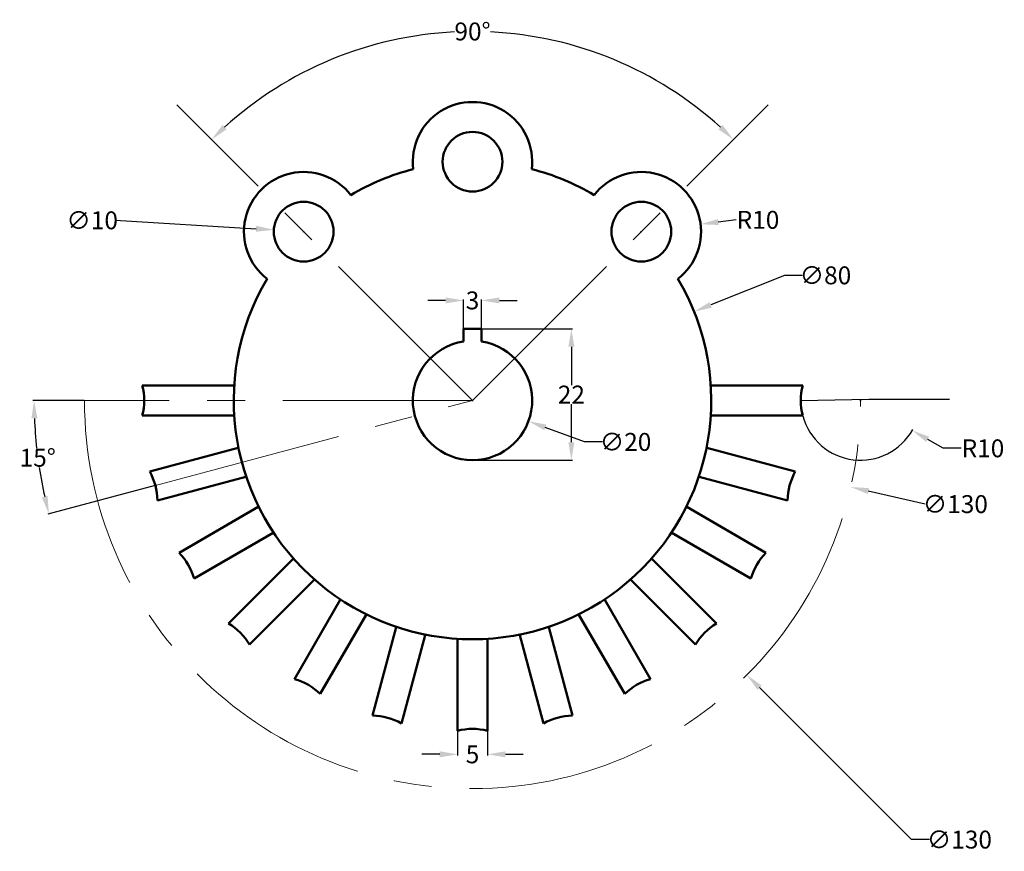
# Model space of a CAD drawing. Units: millimetres. Extents: x 201 to 366, y 129 to 269.
import ezdxf

# ---------------------------------------------------------------- set-up
doc = ezdxf.new("R2010")
doc.units = ezdxf.units.MM
doc.header["$MEASUREMENT"] = 0
doc.linetypes.add('CENTER', pattern=[50.8, 31.75, -6.35, 6.35, -6.35])
for name, color, linetype, lineweight in [('M-CNTR', 1, 'CENTER', 18), ('M-DIMS', 2, 'Continuous', 25), ('M-OUTL', 7, 'Continuous', 50)]:
    doc.layers.add(name, color=color, linetype=linetype, lineweight=lineweight)
doc.styles.get("Standard").update_dxf_attribs({"font": 'arial.ttf'})
doc.dimstyles.get("Standard").update_dxf_attribs({"dimtxt": 3, "dimasz": 3, "dimexe": 0.18, "dimexo": 0.0625, "dimgap": 0.09, "dimtad": 0, "dimtih": 1, "dimtoh": 1, "dimdec": 3, "dimdsep": 46, "dimtxsty": 'Standard', "dimcen": 0.09, "dimadec": 0, "dimazin": 0, "dimtfac": 1, "dimtdec": 3, "dimtofl": 0, "dimtmove": 0, "dimatfit": 3, "dimfxl": 1, "dimtolj": 1, "dimtzin": 0, "dimarcsym": 0})

# ---------------------------------------------------------------- blocks, each defined once
blk = doc.blocks.new('*D1')
at = {"layer": 'Defpoints', "color": 0, "transparency": 16777216}
for p in [(211.72, 204.93), (276.72, 204.93), (276.72, 204.93), (203.54, 198.53), (223.59, 190.7)]:
    blk.add_point(p, dxfattribs=at)
at = {"layer": 'M-DIMS', "color": 0, "lineweight": -2, "transparency": 16777216}
for p, q in [((211.65, 204.93), (203.08, 204.93)), ((223.53, 190.68), (205.59, 185.87))]:
    blk.add_line(p, q, dxfattribs=at)
for start, end in [(182.34, 186.226), (188.7777, 192.66)]:
    blk.add_arc((276.72, 204.93), 73.46, start, end, dxfattribs=at)
at = {"layer": 'M-DIMS', "color": 0, "transparency": 16777216}
for points in [[(202.82, 201.92), (203.82, 201.95), (203.26, 204.93)], [(205.53, 188.95), (204.56, 188.71), (205.76, 185.92)]]:
    blk.add_solid(points, dxfattribs=at)
at = {"layer": 'M-DIMS', "color": 0, "transparency": 16777216, "insert": (203.88, 195.35), "char_height": 3, "attachment_point": 5}
blk.add_mtext('\\A1;15°', dxfattribs=at)
blk = doc.blocks.new('*D2')
at = {"layer": 'Defpoints', "color": 0, "transparency": 16777216}
for p in [(213.35, 219.43), (340.08, 190.44)]:
    blk.add_point(p, dxfattribs=at)
at = {"layer": 'M-DIMS', "color": 0, "lineweight": -2, "transparency": 16777216}
for p, q in [((276.63, 204.93), (276.81, 204.93)), ((276.72, 204.84), (276.72, 205.02)), ((352.57, 187.58), (343, 189.77))]:
    blk.add_line(p, q, dxfattribs=at)
at = {"layer": 'M-DIMS', "color": 0, "transparency": 16777216}
blk.add_solid([(343.12, 190.26), (342.89, 189.28), (340.08, 190.44)], dxfattribs=at)
at = {"layer": 'M-DIMS', "color": 0, "transparency": 16777216, "insert": (357.61, 187.58), "char_height": 3, "attachment_point": 5}
blk.add_mtext('\\A1;∅130', dxfattribs=at)
blk = doc.blocks.new('*D3')
at = {"layer": 'Defpoints', "color": 0, "transparency": 16777216}
for p in [(341.72, 204.93), (350.38, 199.93)]:
    blk.add_point(p, dxfattribs=at)
at = {"layer": 'M-DIMS', "color": 0, "lineweight": -2, "transparency": 16777216}
for p, q in [((341.63, 204.93), (341.81, 204.93)), ((341.72, 204.84), (341.72, 205.02)), ((355.57, 196.93), (352.98, 198.43)), ((358.57, 196.93), (355.57, 196.93))]:
    blk.add_line(p, q, dxfattribs=at)
blk.add_arc((341.72, 204.93), 10, 194.8356, 331.0313, dxfattribs=at)
at = {"layer": 'M-DIMS', "color": 0, "transparency": 16777216}
blk.add_solid([(353.23, 198.87), (352.73, 198), (350.38, 199.93)], dxfattribs=at)
at = {"layer": 'M-DIMS', "color": 0, "transparency": 16777216, "insert": (362.24, 196.93), "char_height": 3, "attachment_point": 5}
blk.add_mtext('\\A1;R10', dxfattribs=at)
blk = doc.blocks.new('*D4')
at = {"layer": 'Defpoints', "color": 0, "transparency": 16777216}
for p in [(274.22, 149.62), (279.22, 149.62), (279.22, 145.67)]:
    blk.add_point(p, dxfattribs=at)
at = {"layer": 'M-DIMS', "color": 0, "lineweight": -2, "transparency": 16777216}
for p, q in [((274.22, 149.55), (274.22, 145.49)), ((279.22, 149.55), (279.22, 145.49)), ((271.22, 145.67), (268.22, 145.67)), ((282.22, 145.67), (285.22, 145.67))]:
    blk.add_line(p, q, dxfattribs=at)
at = {"layer": 'M-DIMS', "color": 0, "transparency": 16777216}
for points in [[(271.22, 146.17), (271.22, 145.17), (274.22, 145.67)], [(282.22, 146.17), (282.22, 145.17), (279.22, 145.67)]]:
    blk.add_solid(points, dxfattribs=at)
at = {"layer": 'M-DIMS', "color": 0, "transparency": 16777216, "insert": (276.72, 145.67), "char_height": 3, "attachment_point": 5}
blk.add_mtext('\\A1;5', dxfattribs=at)
blk = doc.blocks.new('*D5')
at = {"layer": 'Defpoints', "color": 0, "transparency": 16777216}
for p in [(292.72, 264.65), (227.18, 254.47), (326.25, 254.47), (276.72, 204.93), (276.72, 204.93)]:
    blk.add_point(p, dxfattribs=at)
at = {"layer": 'M-DIMS', "color": 0, "lineweight": -2, "transparency": 16777216}
for start, end in [(92.812, 132.2192), (47.7808, 87.188)]:
    blk.add_arc((276.72, 204.93), 61.82, start, end, dxfattribs=at)
at = {"layer": 'M-DIMS', "color": 0, "transparency": 16777216}
for points in [[(235.52, 250.35), (234.83, 251.08), (233.01, 248.65)], [(318.6, 251.08), (317.91, 250.35), (320.43, 248.65)]]:
    blk.add_solid(points, dxfattribs=at)
at = {"layer": 'M-DIMS', "color": 0, "transparency": 16777216, "insert": (276.72, 266.75), "char_height": 3, "attachment_point": 5}
blk.add_mtext('\\A1;90°', dxfattribs=at)
blk = doc.blocks.new('*D6')
at = {"layer": 'Defpoints', "color": 0, "transparency": 16777216}
for p in [(313.84, 219.83), (239.59, 190.04)]:
    blk.add_point(p, dxfattribs=at)
at = {"layer": 'M-DIMS', "color": 0, "lineweight": -2, "transparency": 16777216}
for p, q in [((328.99, 225.9), (316.63, 220.94)), ((331.99, 225.9), (328.99, 225.9)), ((276.63, 204.93), (276.81, 204.93)), ((276.72, 204.84), (276.72, 205.02))]:
    blk.add_line(p, q, dxfattribs=at)
at = {"layer": 'M-DIMS', "color": 0, "transparency": 16777216}
blk.add_solid([(316.44, 221.41), (316.81, 220.48), (313.84, 219.83)], dxfattribs=at)
at = {"layer": 'M-DIMS', "color": 0, "transparency": 16777216, "insert": (335.85, 225.9), "char_height": 3, "attachment_point": 5}
blk.add_mtext('\\A1;∅80', dxfattribs=at)
blk = doc.blocks.new('*D7')
at = {"layer": 'Defpoints', "color": 0, "transparency": 16777216}
for p in [(314.92, 234.46), (305, 233.22)]:
    blk.add_point(p, dxfattribs=at)
at = {"layer": 'M-DIMS', "color": 0, "lineweight": -2, "transparency": 16777216}
for p, q in [((320.88, 235.2), (317.9, 234.83)), ((304.91, 233.22), (305.09, 233.22)), ((305, 233.13), (305, 233.31))]:
    blk.add_line(p, q, dxfattribs=at)
at = {"layer": 'M-DIMS', "color": 0, "transparency": 16777216}
blk.add_solid([(317.84, 235.32), (317.96, 234.33), (314.92, 234.46)], dxfattribs=at)
at = {"layer": 'M-DIMS', "color": 0, "transparency": 16777216, "insert": (324.55, 235.2), "char_height": 3, "attachment_point": 5}
blk.add_mtext('\\A1;R10', dxfattribs=at)
blk = doc.blocks.new('*D8')
at = {"layer": 'Defpoints', "color": 0, "transparency": 16777216}
for p in [(243.44, 233.52), (253.42, 232.92)]:
    blk.add_point(p, dxfattribs=at)
at = {"layer": 'M-DIMS', "color": 0, "lineweight": -2, "transparency": 16777216}
for p, q in [((216.87, 235.12), (240.45, 233.7)), ((248.34, 233.22), (248.52, 233.22)), ((248.43, 233.13), (248.43, 233.31))]:
    blk.add_line(p, q, dxfattribs=at)
at = {"layer": 'M-DIMS', "color": 0, "transparency": 16777216}
blk.add_solid([(240.48, 234.2), (240.42, 233.2), (243.44, 233.52)], dxfattribs=at)
at = {"layer": 'M-DIMS', "color": 0, "transparency": 16777216, "insert": (213, 235.12), "char_height": 3, "attachment_point": 5}
blk.add_mtext('\\A1;∅10', dxfattribs=at)
blk = doc.blocks.new('*D9')
at = {"layer": 'Defpoints', "color": 0, "transparency": 16777216}
for p in [(267.34, 208.4), (286.1, 201.47)]:
    blk.add_point(p, dxfattribs=at)
at = {"layer": 'M-DIMS', "color": 0, "lineweight": -2, "transparency": 16777216}
for p, q in [((276.63, 204.93), (276.81, 204.93)), ((276.72, 204.84), (276.72, 205.02)), ((295.49, 198), (288.91, 200.43)), ((298.49, 198), (295.49, 198))]:
    blk.add_line(p, q, dxfattribs=at)
at = {"layer": 'M-DIMS', "color": 0, "transparency": 16777216}
blk.add_solid([(289.09, 200.9), (288.74, 199.96), (286.1, 201.47)], dxfattribs=at)
at = {"layer": 'M-DIMS', "color": 0, "transparency": 16777216, "insert": (302.36, 198), "char_height": 3, "attachment_point": 5}
blk.add_mtext('\\A1;∅20', dxfattribs=at)
blk = doc.blocks.new('*D10')
at = {"layer": 'Defpoints', "color": 0, "transparency": 16777216}
for p in [(278.22, 221.7), (275.22, 216.93), (278.22, 216.93)]:
    blk.add_point(p, dxfattribs=at)
at = {"layer": 'M-DIMS', "color": 0, "lineweight": -2, "transparency": 16777216}
for p, q in [((272.22, 221.7), (269.22, 221.7)), ((275.22, 217), (275.22, 221.88)), ((278.22, 217), (278.22, 221.88)), ((281.22, 221.7), (284.22, 221.7))]:
    blk.add_line(p, q, dxfattribs=at)
at = {"layer": 'M-DIMS', "color": 0, "transparency": 16777216}
for points in [[(272.22, 222.2), (272.22, 221.2), (275.22, 221.7)], [(281.22, 222.2), (281.22, 221.2), (278.22, 221.7)]]:
    blk.add_solid(points, dxfattribs=at)
at = {"layer": 'M-DIMS', "color": 0, "transparency": 16777216, "insert": (276.72, 221.7), "char_height": 3, "attachment_point": 5}
blk.add_mtext('\\A1;3', dxfattribs=at)
blk = doc.blocks.new('*D11')
at = {"layer": 'Defpoints', "color": 0, "transparency": 16777216}
for p in [(276.71, 216.93), (276.72, 194.93), (293.28, 194.93)]:
    blk.add_point(p, dxfattribs=at)
at = {"layer": 'M-DIMS', "color": 0, "lineweight": -2, "transparency": 16777216}
for p, q in [((276.77, 216.93), (293.46, 216.93)), ((293.28, 213.93), (293.28, 207.53)), ((293.28, 197.93), (293.28, 204.34)), ((276.79, 194.93), (293.46, 194.93))]:
    blk.add_line(p, q, dxfattribs=at)
at = {"layer": 'M-DIMS', "color": 0, "transparency": 16777216}
for points in [[(292.78, 213.93), (293.78, 213.93), (293.28, 216.93)], [(292.78, 197.93), (293.78, 197.93), (293.28, 194.93)]]:
    blk.add_solid(points, dxfattribs=at)
at = {"layer": 'M-DIMS', "color": 0, "transparency": 16777216, "insert": (293.28, 205.93), "char_height": 3, "attachment_point": 5}
blk.add_mtext('\\A1;22', dxfattribs=at)
blk = doc.blocks.new('*D12')
at = {"layer": 'Defpoints', "color": 0, "transparency": 16777216}
for p in [(230.76, 250.9), (322.68, 158.97)]:
    blk.add_point(p, dxfattribs=at)
at = {"layer": 'M-DIMS', "color": 0, "lineweight": -2, "transparency": 16777216}
for p, q in [((276.63, 204.93), (276.81, 204.93)), ((276.72, 204.84), (276.72, 205.02)), ((350.26, 131.39), (324.8, 156.85)), ((353.26, 131.39), (350.26, 131.39))]:
    blk.add_line(p, q, dxfattribs=at)
at = {"layer": 'M-DIMS', "color": 0, "transparency": 16777216}
blk.add_solid([(325.15, 157.2), (324.45, 156.5), (322.68, 158.97)], dxfattribs=at)
at = {"layer": 'M-DIMS', "color": 0, "transparency": 16777216, "insert": (358.29, 131.39), "char_height": 3, "attachment_point": 5}
blk.add_mtext('\\A1;∅130', dxfattribs=at)

msp = doc.modelspace()

# ---------------------------------------------------------------- linework, layer by layer
at = {"layer": 'M-CNTR'}
for p, q in [((276.7172, 204.9343), (227.1825, 254.469)), ((276.7172, 204.9343), (326.2519, 254.469)), ((276.7172, 204.9343), (211.7172, 204.9343)), ((223.5913, 190.6993), (276.7172, 204.9343))]:
    msp.add_line(p, q, dxfattribs=at)
msp.add_arc((276.7172, 204.9343), 65, 180, 0, dxfattribs=at)
at = {"layer": 'M-DIMS'}
for p, q in [((331.7172, 204.9343), (343.1313, 205.1642)), ((343.1313, 205.1642), (356.6517, 205.1642))]:
    msp.add_line(p, q, dxfattribs=at)
at = {"layer": 'M-OUTL'}
for p, q in [((275.2172, 216.9343), (278.2006, 216.9343)), ((275.2172, 214.8212), (275.2172, 216.9343)), ((278.2172, 214.8212), (278.2172, 216.9343)), ((236.7172, 207.4343), (221.3997, 207.4343)), ((236.7172, 207.4343), (221.3997, 207.4343)), ((316.7172, 207.4343), (332.0347, 207.4343)), ((316.7172, 207.4343), (332.0347, 207.4343)), ((236.7172, 202.4343), (221.3997, 202.4343)), ((236.7172, 202.4343), (221.3997, 202.4343)), ((316.7172, 202.4343), (332.0347, 202.4343)), ((237.4331, 196.9964), (222.6375, 193.0319)), ((316.0013, 196.9964), (330.7969, 193.0319)), ((238.7272, 192.1667), (223.9316, 188.2023)), ((314.7072, 192.1667), (329.5028, 188.2023)), ((240.8262, 187.0994), (227.5608, 179.4406)), ((312.6082, 187.0994), (325.8736, 179.4406)), ((243.3262, 182.7693), (230.0608, 175.1105)), ((310.1082, 182.7693), (323.3736, 175.1105)), ((246.6652, 178.4178), (235.834, 167.5867)), ((306.7692, 178.4178), (317.6004, 167.5867)), ((250.2007, 174.8823), (239.3696, 164.0511)), ((303.2337, 174.8823), (314.0648, 164.0511)), ((254.5521, 171.5433), (246.8934, 158.2779)), ((298.8823, 171.5433), (306.541, 158.2779)), ((258.8823, 169.0433), (251.2235, 155.7779)), ((294.5521, 169.0433), (302.2109, 155.7779)), ((263.9496, 166.9443), (259.9852, 152.1487)), ((289.4848, 166.9443), (293.4493, 152.1487)), ((268.7793, 165.6502), (264.8148, 150.8546)), ((284.6552, 165.6502), (288.6196, 150.8546)), ((274.2172, 164.9343), (274.2172, 149.6168)), ((279.2172, 164.9343), (279.2172, 149.6168))]:
    msp.add_line(p, q, dxfattribs=at)
for centre in [(276.7172, 244.9343), (248.4329, 233.2186), (305.0015, 233.2186)]:
    msp.add_circle(centre, 5, dxfattribs=at)
for centre, radius, start, end in [((276.7172, 244.9343), 10, 352.819244, 187.180756), ((248.4329, 233.2186), 10, 37.819244, 232.180756), ((276.7172, 204.9343), 40, 104.361512, 120.638488), ((276.7172, 204.9343), 40, 59.361512, 75.638488), ((305.0015, 233.2186), 10, 307.819244, 142.180756), ((276.7172, 204.9343), 40, 149.361512, 30.638488), ((276.7172, 204.9343), 10, 98.626927, 81.373073), ((211.7172, 204.9343), 10, 345.522488, 14.477512), ((211.7172, 204.9343), 10, 345.522488, 14.477512), ((341.7172, 204.9343), 10, 165.522488, 194.477512), ((341.7172, 204.9343), 10, 165.522488, 194.477512), ((213.932, 188.1111), 10, 0.522488, 29.477512), ((339.5024, 188.1111), 10, 150.522488, 179.477512), ((220.4256, 172.4343), 10, 15.522488, 44.477512), ((333.0089, 172.4343), 10, 135.522488, 164.477512), ((230.7553, 158.9724), 10, 30.522488, 59.477512), ((322.6791, 158.9724), 10, 120.522488, 149.477512), ((244.2172, 148.6427), 10, 45.522488, 74.477512), ((309.2172, 148.6427), 10, 105.522488, 134.477512), ((259.894, 142.1491), 10, 60.522488, 89.477512), ((293.5404, 142.1491), 10, 90.522488, 119.477512), ((276.7172, 139.9343), 10, 75.522488, 104.477512)]:
    msp.add_arc(centre, radius, start, end, dxfattribs=at)

# ---------------------------------------------------------------- dimensions: what is measured, and where the dimension line sits
at = {"layer": 'M-DIMS', "transparency": 33554610}
for base, line1, line2, picture, middle in [((292.7168, 264.6454), ((276.7172, 204.9343), (326.2519, 254.469)), ((276.7172, 204.9343), (227.1825, 254.469)), '*D5', (276.7172, 266.7518)), ((203.5353, 198.5317), ((223.5913, 190.6993), (276.7172, 204.9343)), ((276.7172, 204.9343), (211.7172, 204.9343)), '*D1', (203.8843, 195.3457))]:
    dim = msp.add_angular_dim_2l(base=base, line1=line1, line2=line2, dimstyle='Standard', override={"dimclrd": 0, "dimclre": 0, "dimclrt": 0}, dxfattribs=at)
    dim.commit()
    dim.dimension.update_dxf_attribs({"geometry": picture, "text_midpoint": middle})
at = {"layer": 'M-DIMS'}
dim = msp.add_diameter_dim_2p(p1=(230.756, 250.897), p2=(322.6784, 158.9716), dimstyle='Standard', override={"dimdec": 0, "dimlfac": 1, "dimrnd": 0, "dimzin": 0, "dimdsep": 46, "dimlunit": 2}, dxfattribs=at)
dim.commit()
dim.dimension.update_dxf_attribs({"geometry": '*D12', "text_midpoint": (358.2861, 131.394), "dimtype": 163})
at = {"layer": 'M-DIMS', "transparency": 33554610}
for p1, p2, picture, middle in [((253.4239, 232.9181), (243.442, 233.519), '*D8', (216.8681, 235.1188)), ((239.5933, 190.0409), (313.8411, 219.8278), '*D6', (335.853, 225.9042)), ((213.3542, 219.4303), (340.0802, 190.4383), '*D2', (352.5744, 187.58)), ((267.3366, 208.399), (286.0978, 201.4696), '*D9', (302.3579, 197.9998))]:
    dim = msp.add_diameter_dim_2p(p1=p1, p2=p2, dimstyle='Standard', override={"dimclrd": 0, "dimclre": 0, "dimclrt": 0}, dxfattribs=at)
    dim.commit()
    dim.dimension.update_dxf_attribs({"geometry": picture, "text_midpoint": middle, "dimtype": 163})
for center, mpoint, picture, middle in [((305.0015, 233.2186), (314.9247, 234.4551), '*D7', (324.5478, 235.197)), ((341.7172, 204.9343), (350.3775, 199.9343), '*D3', (362.2427, 196.9343))]:
    dim = msp.add_radius_dim(center=center, mpoint=mpoint, dimstyle='Standard', override={"dimclrd": 0, "dimclre": 0, "dimclrt": 0}, dxfattribs=at)
    dim.commit()
    dim.dimension.update_dxf_attribs({"geometry": picture, "text_midpoint": middle})
for base, p1, p2, picture, middle in [((278.2172, 221.6959), (275.2172, 216.9343), (278.2172, 216.9343), '*D10', (276.7172, 221.6959)), ((279.2172, 145.6704), (274.2172, 149.6168), (279.2172, 149.6168), '*D4', (276.7172, 145.6704))]:
    dim = msp.add_linear_dim(base=base, p1=p1, p2=p2, dimstyle='Standard', override={"dimclrd": 0, "dimclre": 0, "dimclrt": 0}, dxfattribs=at)
    dim.commit()
    dim.dimension.update_dxf_attribs({"geometry": picture, "text_midpoint": middle})
dim = msp.add_linear_dim(base=(293.2753, 194.9343), p1=(276.7089, 216.9343), p2=(276.7241, 194.9343), angle=90, dimstyle='Standard', override={"dimclrd": 0, "dimclre": 0, "dimclrt": 0}, dxfattribs=at)
dim.commit()
dim.dimension.update_dxf_attribs({"geometry": '*D11', "text_midpoint": (293.2753, 205.9343)})

doc.saveas('drawing.dxf')
